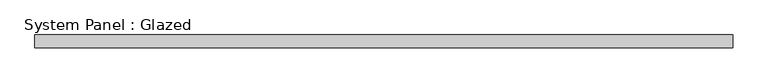
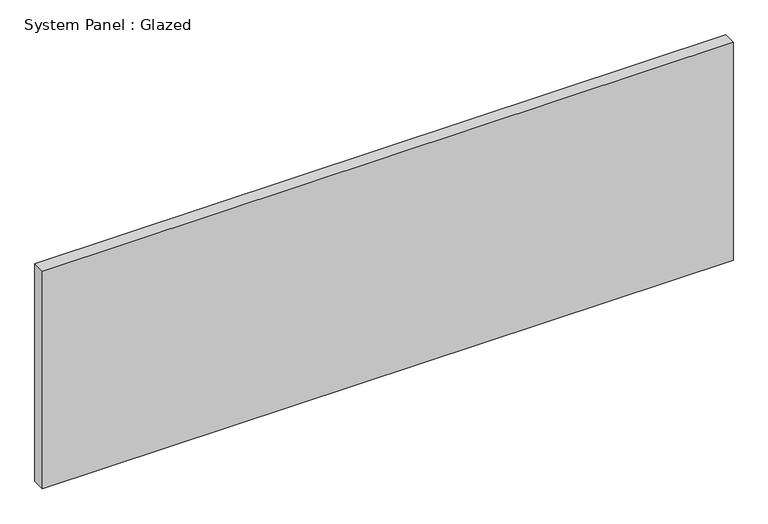
"""IFC4 building model written with IfcOpenShell, lengths in millimetres: plate geometry, System Panel : Glazed."""

from ifc_helpers import new_model, si_unit, origin, origin_with_axes, place, context, project, spatial, polyline, outline, extrude, source, transform, mapped, element, save


def system_panel_glazed_cfd93610(model_context):
    return source(origin(), model_context, "Body", "SweptSolid", [
        extrude(outline(polyline([(685.7999998, -44.45), (-685.7999998, -44.45), (-685.7999998, -19.05), (685.7999998, -19.05), (685.7999998, -44.45)])), origin_with_axes(), (0.0, 0.0, 1.0), 457.2),
    ])


if __name__ == "__main__":
    model = new_model("IFC4")
    model_context = context("Model", 3, world=origin())
    ifc_project = project(units=[si_unit("LENGTHUNIT", "METRE", prefix="MILLI")], contexts=[model_context])
    site = spatial("IfcSite", under=ifc_project)
    building = spatial("IfcBuilding", under=site)
    placement = place(None, origin())
    system_panel_glazed_shape = system_panel_glazed_cfd93610(model_context)
    element("IfcPlate", 1, ObjectType="System Panel : Glazed", at=placement, inside=building, context=model_context, shape_type="MappedRepresentation", body=[
        mapped(system_panel_glazed_shape, transform((0.0, 0.0, 0.0), x_axis=(1.0, 0.0, 0.0), y_axis=(0.0, 1.0, 0.0), z_axis=(0.0, 0.0, 1.0))),
    ])
    save(model, "model.ifc")

# Revit data of these elements
# Type "System Panel : Glazed"
#   Construction Type Id = "GSP4R"
#   Analytic Construction = "1/8 in Pilkington single glazing"
#   Visual Light Transmittance = 0.9
#   Solar Heat Gain Coefficient = 0.86
#   Heat Transfer Coefficient (U) = 1.18115 BTU/(h·ft²·°F)
#   Define Thermal Properties by = 1
# Element 1 (IfcPlate, "System Panel : Glazed")
#   Materials on its faces: "Glass"
# Materials
#   "Glass": class "Glass", colour RGB 0 128 192, transparency 0.75, Description = "Soda Lime Glass", Cost = 0
